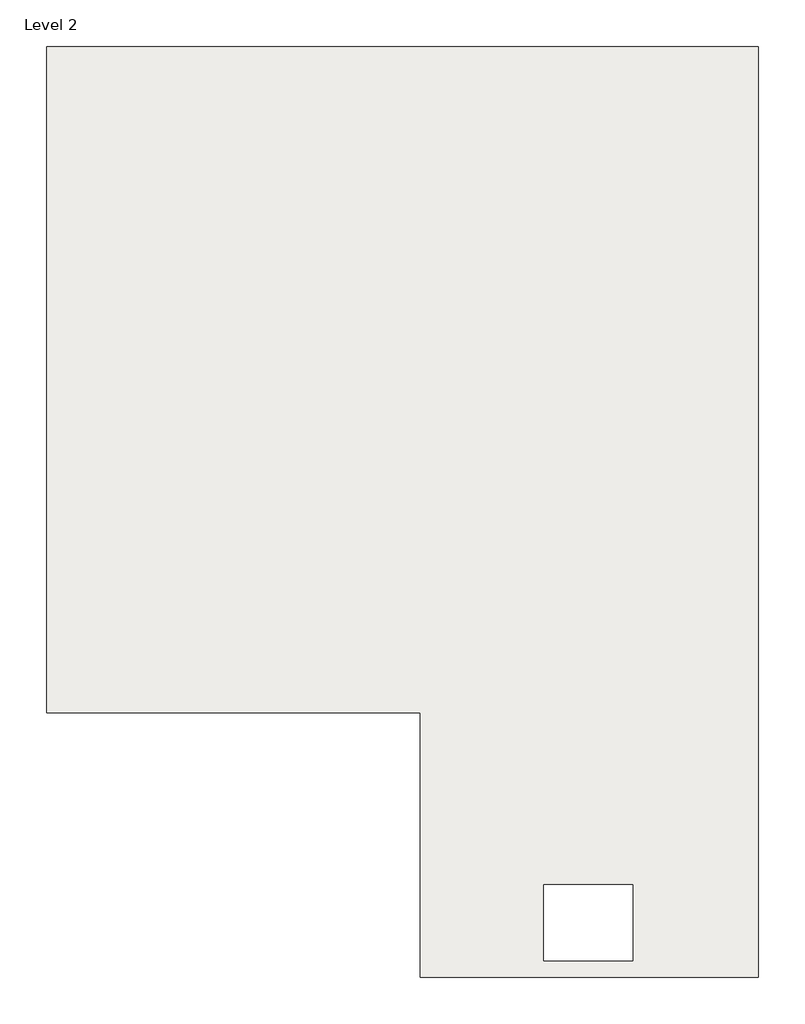
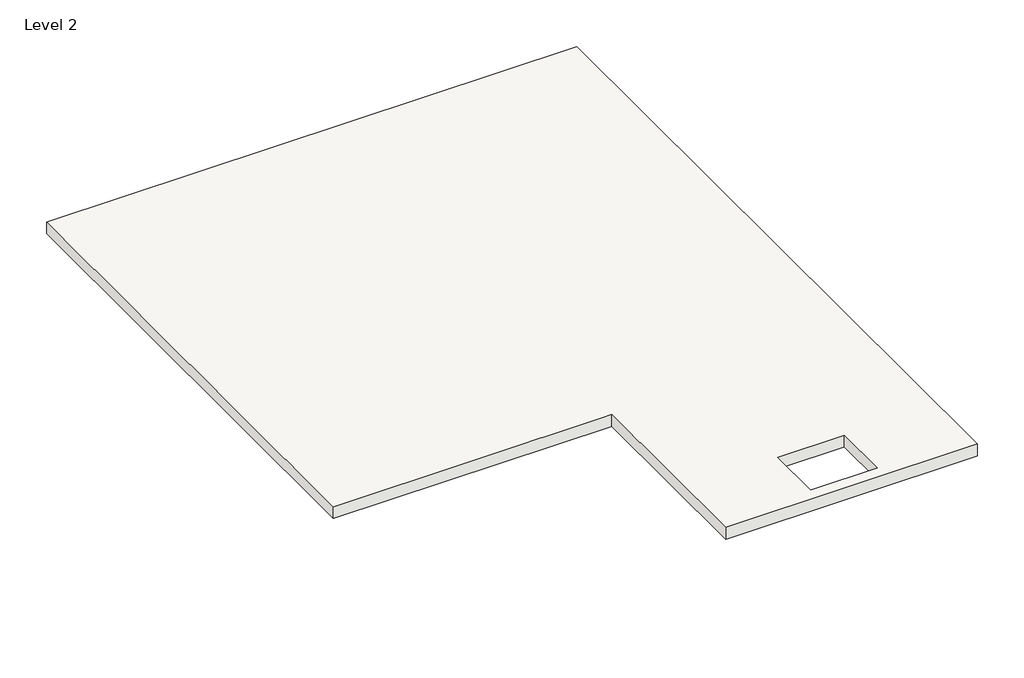
# One storey: 1 roof.
"""IFC4 building model written with IfcOpenShell, lengths in millimetres."""

from ifc_helpers import new_model, si_unit, frame, origin, place, context, project, spatial, polyline, outline, extrude, element, save

model = new_model("IFC4")

# Units and contexts
model_context = context("Model", 3, world=origin())
ifc_project = project(units=[si_unit("LENGTHUNIT", "METRE", prefix="MILLI")], contexts=[model_context])

# Site, building, storey
site = spatial("IfcSite", under=ifc_project)
building = spatial("IfcBuilding", under=site)
storey = spatial("IfcBuildingStorey", under=building, Name="Level 2", Elevation=3048.0)

# Roof
placement = place(None, origin())
element("IfcRoof", 1, ObjectType="Generic - 12\"", at=placement, inside=storey, context=model_context, shape_type="SweptSolid", body=[
    extrude(outline(polyline([(-12707.5816429, 14329.5145179), (338.8064436, 14329.5145179), (338.8064436, -2737.7366944), (-5858.7935564, -2737.7366944), (-5858.7935564, 2113.6633056), (-12707.5816429, 2113.6633056), (-12707.5816429, 14329.5145179)]), holes=[polyline([(-1955.6661463, -2431.9817714), (-1955.6661463, -1034.5333514), (-3587.5741134, -1034.5333514), (-3587.5741134, -2431.9817714), (-1955.6661463, -2431.9817714)])]), frame((0.0, 0.0, 3048.0), z_axis=(0.0, 0.0, 1.0), x_axis=(1.0, 0.0, 0.0)), (0.0, 0.0, 1.0), 304.8),
])

save(model, "model.ifc")

# Revit data of these elements
# Type "Generic - 12\""
#   Assembly Code = "B1020"
#   Layers, outside or top first: 1' - 0" "Brick, Soldier Course" (function 1)
# Element 1 (IfcRoof, "Generic - 12\"")
#   built-in parameter 1001705 = 11 (stored number, unit not read)
#   built-in parameter 1001710 = 33615
#   Phase Created = New Construction
#   Materials on its faces: "Brick, Soldier Course"
# Materials
#   "Brick, Soldier Course": class "Masonry", colour RGB 170 98 104, transparency 0, Description = "Common brick soldier coursed", Cost = 0
